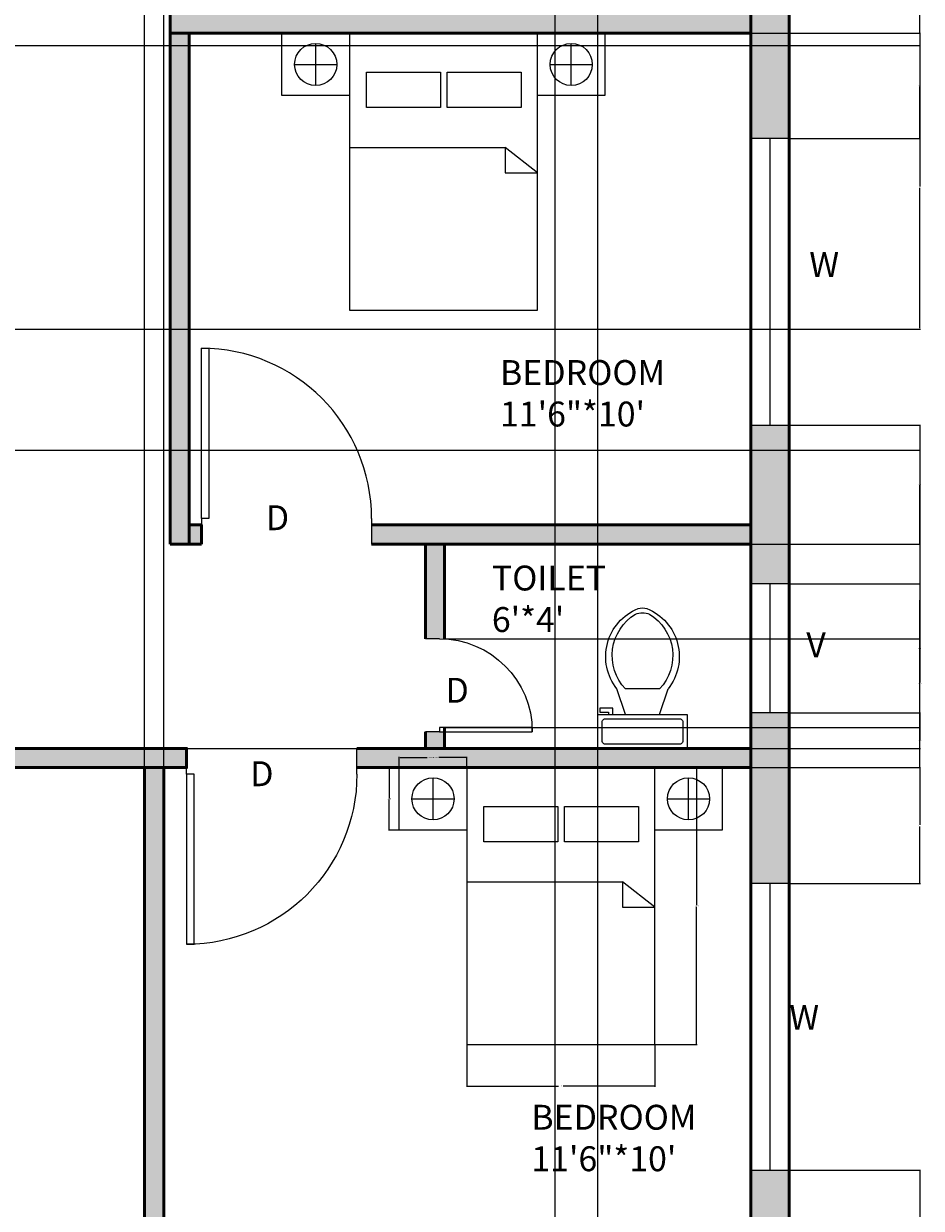
# Model space of a CAD drawing. Units: inches. Extents: x 678 to 1100, y 1432 to 2094.
# Tile 3 of 5: x 889 to 1100, y 1581 to 1860. Entities that reach past the tile are written whole.
import ezdxf

# ---------------------------------------------------------------- set-up
doc = ezdxf.new("R2010")
doc.units = ezdxf.units.IN
for name, color, linetype, lineweight in [('A-ANNO-DIMS', 2, 'Continuous', 18), ('A-AREA-IDEN', 141, 'Continuous', 25), ('A-FLOR-FIXT', 9, 'Continuous', 18), ('A-WALL-PATT', 252, 'Continuous', 13), ('DOOR', 52, 'Continuous', 25), ('FUR', 30, 'Continuous', 18), ('TEXT', 141, 'Continuous', 18), ('WALL', 140, 'Continuous', 50), ('WIND', 212, 'Continuous', 25)]:
    doc.layers.add(name, color=color, linetype=linetype, lineweight=lineweight)
doc.styles.get("Standard").update_dxf_attribs({"font": 'arial.ttf'})
doc.dimstyles.get("Standard").update_dxf_attribs({"dimtxt": 0.18, "dimasz": 0.18, "dimexe": 0.18, "dimexo": 0.0625, "dimgap": 0.09, "dimtad": 0, "dimtih": 1, "dimtoh": 1, "dimdec": 4, "dimzin": 0, "dimdsep": 46, "dimtxsty": 'Standard', "dimcen": 0.09, "dimadec": 0, "dimazin": 0, "dimtfac": 1, "dimtdec": 4, "dimtofl": 0, "dimtmove": 0, "dimatfit": 3, "dimfxl": 1, "dimtolj": 1, "dimtzin": 0, "dimarcsym": 0})

# ---------------------------------------------------------------- blocks, each defined once
blk = doc.blocks.new('*U2')
for p, q in [((0, 0), (0, -6)), ((40, 0), (40, -6))]:
    blk.add_line(p, q)
blk.add_lwpolyline([(0, 0), (0, 40), (1.75, 40), (1.75, 0)], close=True)
blk.add_arc((0, 0), 40, 0, 90)
blk = doc.blocks.new('*U4')
for p, q in [((9.5, -6), (9.5, -2)), ((-8, -8.5), (-8, -8)), ((-7, -8), (-7, -9.5)), ((-4, -8), (-6, -14)), ((4, -8), (6, -14)), ((-10, -8.5), (-8, -8.5)), ((-10, -9.5), (-10, -8.5)), ((-7, -9.5), (-10, -9.5)), ((4, -14), (-4, -14))]:
    blk.add_line(p, q)
blk.add_lwpolyline([(10.5, -8), (10.5, 0), (-10.5, 0), (-10.5, -8)], close=True)
for points in [[(-9.5, -2), (-9.5, -6)], [(8.5, -1), (-8.5, -1)], [(-8.5, -7), (8.5, -7)]]:
    blk.add_lwpolyline(points)
for centre, radius, start, end in [((-8.62, -1.88), 0.884, 81.8699, 188.1301), ((8.62, -1.88), 0.884, 351.8699, 98.1301), ((-8.62, -6.12), 0.884, 171.8699, 278.1301), ((8.62, -6.12), 0.884, 261.8699, 8.1301), ((3.52, -21.58), 12.17, 141.4691, 247.9714), ((4.2, -21.82), 11.33, 136.3677, 238.9468), ((-3.52, -21.58), 12.17, 292.0284, 38.5307), ((-4.2, -21.82), 11.33, 301.053, 43.6321), ((0, -27.88), 4, 245.7318, 294.2682), ((0, -29), 4, 254.8605, 285.1395)]:
    blk.add_arc(centre, radius, start, end)
blk = doc.blocks.new('BED')
for p, q in [((0, 38.19), (36.64, 38.19)), ((36.64, 38.19), (36.64, 32.24)), ((44.21, 32.24), (36.64, 38.19)), ((36.64, 32.24), (44.21, 32.24))]:
    blk.add_line(p, q)
for points in [[(44.21, 65.05), (0, 65.05), (0, 0), (44.21, 0)], [(4.01, 55.91), (21.41, 55.91), (21.41, 47.59), (4.01, 47.59)], [(22.97, 55.91), (40.37, 55.91), (40.37, 47.59), (22.97, 47.59)]]:
    blk.add_lwpolyline(points, close=True)
blk = doc.blocks.new('NIGHTSTAND-LAMP')
for p, q in [((7.92, 2.38), (7.92, 12.28)), ((2.97, 7.33), (12.87, 7.33))]:
    blk.add_line(p, q)
blk.add_lwpolyline([(0, 14.65), (15.83, 14.65), (15.83, 0), (0, 0)], close=True)
blk.add_circle((7.92, 7.33), 4.95)
blk = doc.blocks.new('WIN-STANDARD')
blk.add_line((4.5, 0), (4.5, 67.31))
blk.add_lwpolyline([(9, 67.31), (0, 67.31), (0, 0), (9, 0)], close=True)
blk = doc.blocks.new('*D14')
at = {"layer": 'A-ANNO-DIMS', "color": 0, "lineweight": -2, "transparency": 16777216}
for p, q in [((1037.43, 1684.93), (1047.3, 1684.93)), ((1047.12, 1684.75), (1047.12, 1652.59)), ((1047.12, 1620.06), (1047.12, 1652.22)), ((1037.43, 1619.88), (1047.3, 1619.88))]:
    blk.add_line(p, q, dxfattribs=at)
at = {"layer": 'A-ANNO-DIMS', "color": 0, "transparency": 16777216}
for points in [[(1047.09, 1684.75), (1047.15, 1684.75), (1047.12, 1684.93)], [(1047.09, 1620.06), (1047.15, 1620.06), (1047.12, 1619.88)]]:
    blk.add_solid(points, dxfattribs=at)
at = {"layer": 'Defpoints', "color": 0, "transparency": 16777216}
for p in [(1037.36, 1684.93), (1047.12, 1684.93), (1037.36, 1619.88)]:
    blk.add_point(p, dxfattribs=at)
at = {"layer": 'A-ANNO-DIMS', "color": 0, "transparency": 16777216, "insert": (1047.12, 1652.4), "char_height": 0.18, "attachment_point": 5}
blk.add_mtext('\\A1;BED 65 TYP.', dxfattribs=at)
blk = doc.blocks.new('*D15')
at = {"layer": 'A-ANNO-DIMS', "color": 0, "lineweight": -2, "transparency": 16777216}
for p, q in [((993.15, 1619.82), (993.15, 1609.94)), ((1037.36, 1619.82), (1037.36, 1609.94)), ((993.33, 1610.12), (1014.72, 1610.12)), ((1037.18, 1610.12), (1015.79, 1610.12))]:
    blk.add_line(p, q, dxfattribs=at)
at = {"layer": 'A-ANNO-DIMS', "color": 0, "transparency": 16777216}
for points in [[(993.33, 1610.15), (993.33, 1610.09), (993.15, 1610.12)], [(1037.18, 1610.15), (1037.18, 1610.09), (1037.36, 1610.12)]]:
    blk.add_solid(points, dxfattribs=at)
at = {"layer": 'Defpoints', "color": 0, "transparency": 16777216}
for p in [(993.15, 1619.88), (1037.36, 1619.88), (1037.36, 1610.12)]:
    blk.add_point(p, dxfattribs=at)
at = {"layer": 'A-ANNO-DIMS', "color": 0, "transparency": 16777216, "insert": (1015.26, 1610.12), "char_height": 0.18, "attachment_point": 5}
blk.add_mtext('\\A1;44 TYP.', dxfattribs=at)
blk = doc.blocks.new('*D16')
at = {"layer": 'A-ANNO-DIMS', "color": 0, "lineweight": -2, "transparency": 16777216}
for p, q in [((977.31, 1684.99), (977.31, 1687.48)), ((977.49, 1687.3), (983.86, 1687.3)), ((992.97, 1687.3), (986.61, 1687.3)), ((993.15, 1684.99), (993.15, 1687.48))]:
    blk.add_line(p, q, dxfattribs=at)
at = {"layer": 'A-ANNO-DIMS', "color": 0, "transparency": 16777216}
for points in [[(977.49, 1687.33), (977.49, 1687.27), (977.31, 1687.3)], [(992.97, 1687.33), (992.97, 1687.27), (993.15, 1687.3)]]:
    blk.add_solid(points, dxfattribs=at)
at = {"layer": 'Defpoints', "color": 0, "transparency": 16777216}
for p in [(993.15, 1687.3), (977.31, 1684.93), (993.15, 1684.93)]:
    blk.add_point(p, dxfattribs=at)
at = {"layer": 'A-ANNO-DIMS', "color": 0, "transparency": 16777216, "insert": (985.23, 1687.3), "char_height": 0.18, "attachment_point": 5}
blk.add_mtext('\\A1;NIGHTSTAND 16 TYP.', dxfattribs=at)
blk = doc.blocks.new('*D17')
at = {"layer": 'A-ANNO-DIMS', "color": 0, "lineweight": -2, "transparency": 16777216}
for p, q in [((977.25, 1684.93), (974.76, 1684.93)), ((974.94, 1684.75), (974.94, 1677.78)), ((974.94, 1670.45), (974.94, 1677.42)), ((977.25, 1670.27), (974.76, 1670.27))]:
    blk.add_line(p, q, dxfattribs=at)
at = {"layer": 'A-ANNO-DIMS', "color": 0, "transparency": 16777216}
for points in [[(974.91, 1684.75), (974.97, 1684.75), (974.94, 1684.93)], [(974.91, 1670.45), (974.97, 1670.45), (974.94, 1670.27)]]:
    blk.add_solid(points, dxfattribs=at)
at = {"layer": 'Defpoints', "color": 0, "transparency": 16777216}
for p in [(974.94, 1684.93), (977.31, 1684.93), (977.31, 1670.27)]:
    blk.add_point(p, dxfattribs=at)
at = {"layer": 'A-ANNO-DIMS', "color": 0, "transparency": 16777216, "insert": (974.94, 1677.6), "char_height": 0.18, "attachment_point": 5}
blk.add_mtext('\\A1;15 TYP.', dxfattribs=at)
blk = doc.blocks.new('*D33')
at = {"layer": 'A-ANNO-DIMS', "color": 0, "lineweight": -2, "transparency": 16777216}
for p, q in [((1069.02, 1590.39), (1099.79, 1590.39)), ((1099.61, 1590.21), (1099.61, 1575.59)), ((1099.61, 1560.61), (1099.61, 1575.23)), ((1069.02, 1560.43), (1099.79, 1560.43))]:
    blk.add_line(p, q, dxfattribs=at)
at = {"layer": 'A-ANNO-DIMS', "color": 0, "transparency": 16777216}
for points in [[(1099.58, 1590.21), (1099.64, 1590.21), (1099.61, 1590.39)], [(1099.58, 1560.61), (1099.64, 1560.61), (1099.61, 1560.43)]]:
    blk.add_solid(points, dxfattribs=at)
at = {"layer": 'Defpoints', "color": 0, "transparency": 16777216}
for p in [(1068.96, 1590.39), (1099.61, 1590.39), (1068.96, 1560.43)]:
    blk.add_point(p, dxfattribs=at)
at = {"layer": 'A-ANNO-DIMS', "color": 0, "transparency": 16777216, "insert": (1099.61, 1575.41), "char_height": 0.18, "attachment_point": 5}
blk.add_mtext('\\A1;29.96', dxfattribs=at)
blk = doc.blocks.new('*D34')
at = {"layer": 'A-ANNO-DIMS', "color": 0, "lineweight": -2, "transparency": 16777216}
for p, q in [((1060.02, 1684.93), (1099.79, 1684.93)), ((1099.61, 1684.75), (1099.61, 1671.5)), ((1099.61, 1657.88), (1099.61, 1671.13)), ((1069.02, 1657.7), (1099.79, 1657.7))]:
    blk.add_line(p, q, dxfattribs=at)
at = {"layer": 'A-ANNO-DIMS', "color": 0, "transparency": 16777216}
for points in [[(1099.58, 1684.75), (1099.64, 1684.75), (1099.61, 1684.93)], [(1099.58, 1657.88), (1099.64, 1657.88), (1099.61, 1657.7)]]:
    blk.add_solid(points, dxfattribs=at)
at = {"layer": 'Defpoints', "color": 0, "transparency": 16777216}
for p in [(1059.96, 1684.93), (1099.61, 1684.93), (1068.96, 1657.7)]:
    blk.add_point(p, dxfattribs=at)
at = {"layer": 'A-ANNO-DIMS', "color": 0, "transparency": 16777216, "insert": (1099.61, 1671.32), "char_height": 0.18, "attachment_point": 5}
blk.add_mtext('\\A1;27.227', dxfattribs=at)
blk = doc.blocks.new('*D35')
at = {"layer": 'A-ANNO-DIMS', "color": 0, "lineweight": -2, "transparency": 16777216}
for p, q in [((1069.02, 1697.8), (1099.79, 1697.8)), ((1099.61, 1697.62), (1099.61, 1691.55)), ((1099.61, 1685.11), (1099.61, 1691.18)), ((1060.02, 1684.93), (1099.79, 1684.93))]:
    blk.add_line(p, q, dxfattribs=at)
at = {"layer": 'A-ANNO-DIMS', "color": 0, "transparency": 16777216}
for points in [[(1099.58, 1697.62), (1099.64, 1697.62), (1099.61, 1697.8)], [(1099.58, 1685.11), (1099.64, 1685.11), (1099.61, 1684.93)]]:
    blk.add_solid(points, dxfattribs=at)
at = {"layer": 'Defpoints', "color": 0, "transparency": 16777216}
for p in [(1068.96, 1697.8), (1099.61, 1697.8), (1059.96, 1684.93)]:
    blk.add_point(p, dxfattribs=at)
at = {"layer": 'A-ANNO-DIMS', "color": 0, "transparency": 16777216, "insert": (1099.61, 1691.37), "char_height": 0.18, "attachment_point": 5}
blk.add_mtext('\\A1;12.873', dxfattribs=at)
blk = doc.blocks.new('*D36')
at = {"layer": 'A-ANNO-DIMS', "color": 0, "lineweight": -2, "transparency": 16777216}
for p, q in [((1069.02, 1728.14), (1099.79, 1728.14)), ((1099.61, 1727.96), (1099.61, 1713.16)), ((1099.61, 1697.98), (1099.61, 1712.79)), ((1069.02, 1697.8), (1099.79, 1697.8))]:
    blk.add_line(p, q, dxfattribs=at)
at = {"layer": 'A-ANNO-DIMS', "color": 0, "transparency": 16777216}
for points in [[(1099.58, 1727.96), (1099.64, 1727.96), (1099.61, 1728.14)], [(1099.58, 1697.98), (1099.64, 1697.98), (1099.61, 1697.8)]]:
    blk.add_solid(points, dxfattribs=at)
at = {"layer": 'Defpoints', "color": 0, "transparency": 16777216}
for p in [(1068.96, 1728.14), (1099.61, 1728.14), (1068.96, 1697.8)]:
    blk.add_point(p, dxfattribs=at)
at = {"layer": 'A-ANNO-DIMS', "color": 0, "transparency": 16777216, "insert": (1099.61, 1712.97), "char_height": 0.18, "attachment_point": 5}
blk.add_mtext('\\A1;30.34', dxfattribs=at)
blk = doc.blocks.new('*D37')
at = {"layer": 'A-ANNO-DIMS', "color": 0, "lineweight": -2, "transparency": 16777216}
for p, q in [((1069.02, 1765.41), (1099.79, 1765.41)), ((1099.61, 1765.23), (1099.61, 1751.6)), ((1099.61, 1737.61), (1099.61, 1751.24)), ((1060.02, 1737.43), (1099.79, 1737.43))]:
    blk.add_line(p, q, dxfattribs=at)
at = {"layer": 'A-ANNO-DIMS', "color": 0, "transparency": 16777216}
for points in [[(1099.58, 1765.23), (1099.64, 1765.23), (1099.61, 1765.41)], [(1099.58, 1737.61), (1099.64, 1737.61), (1099.61, 1737.43)]]:
    blk.add_solid(points, dxfattribs=at)
at = {"layer": 'Defpoints', "color": 0, "transparency": 16777216}
for p in [(1068.96, 1765.41), (1099.61, 1765.41), (1059.96, 1737.43)]:
    blk.add_point(p, dxfattribs=at)
at = {"layer": 'A-ANNO-DIMS', "color": 0, "transparency": 16777216, "insert": (1099.61, 1751.42), "char_height": 0.18, "attachment_point": 5}
blk.add_mtext('\\A1;27.98', dxfattribs=at)
blk = doc.blocks.new('*D38')
at = {"layer": 'A-ANNO-DIMS', "color": 0, "lineweight": -2, "transparency": 16777216}
for p, q in [((1060.02, 1857.43), (1099.79, 1857.43)), ((1099.61, 1857.25), (1099.61, 1845.25)), ((1099.61, 1832.9), (1099.61, 1844.89)), ((1069.02, 1832.72), (1099.79, 1832.72))]:
    blk.add_line(p, q, dxfattribs=at)
at = {"layer": 'A-ANNO-DIMS', "color": 0, "transparency": 16777216}
for points in [[(1099.58, 1857.25), (1099.64, 1857.25), (1099.61, 1857.43)], [(1099.58, 1832.9), (1099.64, 1832.9), (1099.61, 1832.72)]]:
    blk.add_solid(points, dxfattribs=at)
at = {"layer": 'Defpoints', "color": 0, "transparency": 16777216}
for p in [(1059.96, 1857.43), (1099.61, 1857.43), (1068.96, 1832.72)]:
    blk.add_point(p, dxfattribs=at)
at = {"layer": 'A-ANNO-DIMS', "color": 0, "transparency": 16777216, "insert": (1099.61, 1845.07), "char_height": 0.18, "attachment_point": 5}
blk.add_mtext('\\A1;24.71', dxfattribs=at)
blk = doc.blocks.new('*D39')
at = {"layer": 'A-ANNO-DIMS', "color": 0, "lineweight": -2, "transparency": 16777216}
for p, q in [((1069.02, 1935.32), (1099.79, 1935.32)), ((1099.61, 1935.14), (1099.61, 1896.56)), ((1099.61, 1857.61), (1099.61, 1896.19)), ((1060.02, 1857.43), (1099.79, 1857.43))]:
    blk.add_line(p, q, dxfattribs=at)
at = {"layer": 'A-ANNO-DIMS', "color": 0, "transparency": 16777216}
for points in [[(1099.58, 1935.14), (1099.64, 1935.14), (1099.61, 1935.32)], [(1099.58, 1857.61), (1099.64, 1857.61), (1099.61, 1857.43)]]:
    blk.add_solid(points, dxfattribs=at)
at = {"layer": 'Defpoints', "color": 0, "transparency": 16777216}
for p in [(1068.96, 1935.32), (1099.61, 1935.32), (1059.96, 1857.43)]:
    blk.add_point(p, dxfattribs=at)
at = {"layer": 'A-ANNO-DIMS', "color": 0, "transparency": 16777216, "insert": (1099.61, 1896.38), "char_height": 0.18, "attachment_point": 5}
blk.add_mtext('\\A1;77.9', dxfattribs=at)
blk = doc.blocks.new('*D41')
at = {"layer": 'A-ANNO-DIMS', "color": 0, "lineweight": -2, "transparency": 16777216}
for p, q in [((718.02, 1759.52), (1099.79, 1759.52)), ((1099.61, 1759.34), (1099.61, 1724.66)), ((1099.61, 1689.61), (1099.61, 1724.29)), ((718.02, 1689.43), (1099.79, 1689.43))]:
    blk.add_line(p, q, dxfattribs=at)
at = {"layer": 'A-ANNO-DIMS', "color": 0, "transparency": 16777216}
for points in [[(1099.58, 1759.34), (1099.64, 1759.34), (1099.61, 1759.52)], [(1099.58, 1689.61), (1099.64, 1689.61), (1099.61, 1689.43)]]:
    blk.add_solid(points, dxfattribs=at)
at = {"layer": 'Defpoints', "color": 0, "transparency": 16777216}
for p in [(717.96, 1759.52), (1099.61, 1759.52), (717.96, 1689.43)]:
    blk.add_point(p, dxfattribs=at)
at = {"layer": 'A-ANNO-DIMS', "color": 0, "transparency": 16777216, "insert": (1099.61, 1724.48), "char_height": 0.18, "attachment_point": 5}
blk.add_mtext('\\A1;70.1', dxfattribs=at)
blk = doc.blocks.new('*D46')
at = {"layer": 'A-ANNO-DIMS', "color": 0, "lineweight": -2, "transparency": 16777216}
for p, q in [((988.02, 1715.16), (1099.79, 1715.16)), ((1099.61, 1714.98), (1099.61, 1704.92)), ((1099.61, 1694.5), (1099.61, 1704.56)), ((988.02, 1694.32), (1099.79, 1694.32))]:
    blk.add_line(p, q, dxfattribs=at)
at = {"layer": 'A-ANNO-DIMS', "color": 0, "transparency": 16777216}
for points in [[(1099.58, 1714.98), (1099.64, 1714.98), (1099.61, 1715.16)], [(1099.58, 1694.5), (1099.64, 1694.5), (1099.61, 1694.32)]]:
    blk.add_solid(points, dxfattribs=at)
at = {"layer": 'Defpoints', "color": 0, "transparency": 16777216}
for p in [(987.96, 1715.16), (1099.61, 1715.16), (987.96, 1694.32)]:
    blk.add_point(p, dxfattribs=at)
at = {"layer": 'A-ANNO-DIMS', "color": 0, "transparency": 16777216, "insert": (1099.61, 1704.74), "char_height": 0.18, "attachment_point": 5}
blk.add_mtext('\\A1;20.844', dxfattribs=at)
blk = doc.blocks.new('*D48')
at = {"layer": 'A-ANNO-DIMS', "color": 0, "lineweight": -2, "transparency": 16777216}
for p, q in [((917.46, 1560.49), (917.46, 2093.76)), ((917.64, 2093.58), (919.45, 2093.58)), ((921.78, 2093.58), (919.97, 2093.58)), ((921.96, 1560.49), (921.96, 2093.76))]:
    blk.add_line(p, q, dxfattribs=at)
at = {"layer": 'A-ANNO-DIMS', "color": 0, "transparency": 16777216}
for points in [[(917.64, 2093.61), (917.64, 2093.55), (917.46, 2093.58)], [(921.78, 2093.61), (921.78, 2093.55), (921.96, 2093.58)]]:
    blk.add_solid(points, dxfattribs=at)
at = {"layer": 'Defpoints', "color": 0, "transparency": 16777216}
for p in [(921.96, 2093.58), (917.46, 1560.43), (921.96, 1560.43)]:
    blk.add_point(p, dxfattribs=at)
at = {"layer": 'A-ANNO-DIMS', "color": 0, "transparency": 16777216, "insert": (919.71, 2093.58), "char_height": 0.18, "attachment_point": 5}
blk.add_mtext('\\A1;4.5', dxfattribs=at)
blk = doc.blocks.new('*D49')
at = {"layer": 'A-ANNO-DIMS', "color": 0, "lineweight": -2, "transparency": 16777216}
for p, q in [((1013.96, 1471.99), (1013.96, 2093.76)), ((1014.14, 2093.58), (1018.75, 2093.58)), ((1023.78, 2093.58), (1019.17, 2093.58)), ((1023.96, 1471.99), (1023.96, 2093.76))]:
    blk.add_line(p, q, dxfattribs=at)
at = {"layer": 'A-ANNO-DIMS', "color": 0, "transparency": 16777216}
for points in [[(1014.14, 2093.61), (1014.14, 2093.55), (1013.96, 2093.58)], [(1023.78, 2093.61), (1023.78, 2093.55), (1023.96, 2093.58)]]:
    blk.add_solid(points, dxfattribs=at)
at = {"layer": 'Defpoints', "color": 0, "transparency": 16777216}
for p in [(1023.96, 2093.58), (1013.96, 1471.93), (1023.96, 1471.93)]:
    blk.add_point(p, dxfattribs=at)
at = {"layer": 'A-ANNO-DIMS', "color": 0, "transparency": 16777216, "insert": (1018.96, 2093.58), "char_height": 0.18, "attachment_point": 5}
blk.add_mtext('\\A1;10', dxfattribs=at)
blk = doc.blocks.new('*D50')
at = {"layer": 'A-ANNO-DIMS', "color": 0, "lineweight": -2, "transparency": 16777216}
for p, q in [((1023.96, 1471.99), (1023.96, 2093.76)), ((1024.14, 2093.58), (1041.74, 2093.58)), ((1059.78, 2093.58), (1042.18, 2093.58)), ((1059.96, 1471.99), (1059.96, 2093.76))]:
    blk.add_line(p, q, dxfattribs=at)
at = {"layer": 'A-ANNO-DIMS', "color": 0, "transparency": 16777216}
for points in [[(1024.14, 2093.61), (1024.14, 2093.55), (1023.96, 2093.58)], [(1059.78, 2093.61), (1059.78, 2093.55), (1059.96, 2093.58)]]:
    blk.add_solid(points, dxfattribs=at)
at = {"layer": 'Defpoints', "color": 0, "transparency": 16777216}
for p in [(1059.96, 2093.58), (1023.96, 1471.93), (1059.96, 1471.93)]:
    blk.add_point(p, dxfattribs=at)
at = {"layer": 'A-ANNO-DIMS', "color": 0, "transparency": 16777216, "insert": (1041.96, 2093.58), "char_height": 0.18, "attachment_point": 5}
blk.add_mtext('\\A1;36', dxfattribs=at)
blk = doc.blocks.new('*D56')
at = {"layer": 'A-ANNO-DIMS', "color": 0, "lineweight": -2, "transparency": 16777216}
for p, q in [((720.28, 1854.56), (1099.79, 1854.56)), ((1099.61, 1854.38), (1099.61, 1821.43)), ((1099.61, 1788.12), (1099.61, 1821.06)), ((720.28, 1787.94), (1099.79, 1787.94))]:
    blk.add_line(p, q, dxfattribs=at)
at = {"layer": 'A-ANNO-DIMS', "color": 0, "transparency": 16777216}
for points in [[(1099.58, 1854.38), (1099.64, 1854.38), (1099.61, 1854.56)], [(1099.58, 1788.12), (1099.64, 1788.12), (1099.61, 1787.94)]]:
    blk.add_solid(points, dxfattribs=at)
at = {"layer": 'Defpoints', "color": 0, "transparency": 16777216}
for p in [(720.22, 1854.56), (1099.61, 1854.56), (720.22, 1787.94)]:
    blk.add_point(p, dxfattribs=at)
at = {"layer": 'A-ANNO-DIMS', "color": 0, "transparency": 16777216, "insert": (1099.61, 1821.25), "char_height": 0.18, "attachment_point": 5}
blk.add_mtext('\\A1;66.62', dxfattribs=at)

msp = doc.modelspace()

# ---------------------------------------------------------------- hatches: boundary and pattern name
at = {"layer": 'A-WALL-PATT'}
h = msp.add_hatch(color=256, dxfattribs=at)
h.dxf.hatch_style = 1
h.paths.add_polyline_path([(859.7133, 2062.9286), (708.9606, 2062.9286), (708.9606, 2031.3203), (717.9606, 2031.3203), (717.9606, 2053.9286), (837.9606, 2053.9286), (859.7133, 2053.9286)])
h.paths.add_polyline_path([(957.0069, 2062.9286), (896.0724, 2062.9286), (896.0724, 2053.9286), (957.0069, 2053.9286)])
h.paths.add_polyline_path([(842.4606, 2053.9286), (837.9606, 2053.9286), (837.9606, 2005.4286), (842.4606, 2005.4286), (923.4606, 2005.4286), (923.4606, 2009.9286), (842.4606, 2009.9286)])
h.paths.add_polyline_path([(927.9606, 2053.9286), (923.4606, 2053.9286), (923.4606, 2052.1286), (924.8103, 2052.1286), (927.9606, 2052.1286)])
h.paths.add_polyline_path([(1068.9606, 2062.9286), (1024.3184, 2062.9286), (1024.3184, 2053.9286), (1028.6041, 2053.9286), (1059.9606, 2053.9286), (1059.9606, 2002.6361), (1068.9606, 2002.6361)])
h.paths.add_polyline_path([(1059.9606, 1861.9286), (996.9604, 1861.9286), (927.9606, 1861.9286), (923.4606, 1861.9286), (923.4606, 1857.4286), (1059.9606, 1857.4286)], flags=17)
h.paths.add_polyline_path([(927.9606, 2031.1269), (924.8103, 2031.1269, -0.01607952), (923.4606, 2031.1703), (923.4606, 1905.3856), (927.9606, 1905.3856)])
h.paths.add_polyline_path([(923.4606, 1957.9286), (842.4606, 1957.9286), (842.4606, 1969.339), (837.9606, 1969.339), (837.9606, 1953.4286), (923.4606, 1953.4286)])
h.paths.add_polyline_path([(774.6357, 1957.9286), (717.9606, 1957.9286), (717.9606, 1953.4286), (774.6357, 1953.4286)])
h.paths.add_polyline_path([(717.9606, 1979.9404), (708.9606, 1979.9404), (708.9606, 1945.1463), (717.9606, 1945.1463)])
h.paths.add_polyline_path([(840.5596, 1861.9286), (717.9606, 1861.9286), (717.9606, 1857.4286), (840.5596, 1857.4286)], flags=17)
h.paths.add_polyline_path([(927.9606, 1865.3856), (923.4606, 1865.3856), (923.4606, 1861.9286), (927.9606, 1861.9286)], flags=17)
h.paths.add_polyline_path([(1059.9606, 1689.4286), (967.3461, 1689.4286), (967.3461, 1684.9286), (1059.9606, 1684.9286)], flags=17)
h.paths.add_polyline_path([(987.9606, 1737.4286), (983.4606, 1737.4286), (983.4606, 1715.196), (986.7357, 1715.196, -0.01403382), (987.9606, 1715.1616)], flags=17)
h.paths.add_polyline_path([(916.0499, 2036.8414), (924.8721, 2036.8414), (924.8721, 2048.8901), (916.0499, 2048.8901)], flags=9)
h.paths.add_polyline_path([(921.7778, 1883.2914), (930.5999, 1883.2914), (930.5999, 1895.3401), (921.7778, 1895.3401)], flags=25)
h.paths.add_polyline_path([(732.1085, 1683.0506), (740.9307, 1683.0506), (740.9307, 1695.0993), (732.1085, 1695.0993)], flags=25)
h.paths.add_polyline_path([(943.8458, 1737.5114), (952.6679, 1737.5114), (952.6679, 1749.5601), (943.8458, 1749.5601)], flags=25)
h.paths.add_polyline_path([(986.0751, 1696.9795), (994.8973, 1696.9795), (994.8973, 1709.0282), (986.0751, 1709.0282)], flags=25)
h.paths.add_polyline_path([(940.1881, 1677.378), (949.0103, 1677.378), (949.0103, 1689.4267), (940.1881, 1689.4267)], flags=25)
h.paths.add_polyline_path([(998.6262, 1761.7469), (1044.0453, 1761.7469), (1044.0453, 1783.5644), (998.6262, 1783.5644)], flags=25)
h.paths.add_polyline_path([(997.3001, 1713.4735), (1028.9316, 1713.4735), (1028.9316, 1735.2909), (997.3001, 1735.2909)], flags=25)
h.paths.add_polyline_path([(1005.9896, 1586.8139), (1051.4087, 1586.8139), (1051.4087, 1608.6313), (1005.9896, 1608.6313)], flags=25)
h.paths.add_polyline_path([(794.7038, 1552.8124), (873.8721, 1552.8124), (873.8721, 1574.6298), (794.7038, 1574.6298)], flags=25)
h.paths.add_polyline_path([(774.2693, 1771.1228), (831.9444, 1771.1228), (831.9444, 1792.9403), (774.2693, 1792.9403)], flags=25)
h.paths.add_polyline_path([(750.0357, 1897.1514), (786.4291, 1897.1514), (786.4291, 1918.9689), (750.0357, 1918.9689)], flags=25)
h.paths.add_polyline_path([(974.9086, 1953.7921), (1020.3276, 1953.7921), (1020.3276, 1975.6096), (974.9086, 1975.6096)], flags=9)
h.paths.add_polyline_path([(859.1564, 1973.8092), (890.2175, 1973.8092), (890.2175, 1995.6267), (859.1564, 1995.6267)], flags=9)
h.paths.add_polyline_path([(753.2305, 1989.0219), (792.2962, 1989.0219), (792.2962, 2010.8393), (753.2305, 2010.8393)], flags=9)
h.paths.add_polyline_path([(1067.3992, 1620.1515), (1078.032, 1620.1515), (1078.032, 1632.2002), (1067.3992, 1632.2002)], flags=9)
h.paths.add_polyline_path([(846.8446, 2028.8178), (878.5079, 2028.8178), (878.5079, 2050.6353), (846.8446, 2050.6353)], flags=25)
h.paths.add_polyline_path([(1059.9606, 1832.7202), (1068.9606, 1832.7202), (1068.9606, 1935.3246), (1059.9606, 1935.3246)])
h.paths.add_polyline_path([(1068.9606, 1765.4088), (1059.9606, 1765.4088), (1059.9606, 1728.1446), (1068.9606, 1728.1446)])
h.paths.add_polyline_path([(1059.9606, 1657.7018), (1068.9606, 1657.7018), (1068.9606, 1697.8017), (1059.9606, 1697.8017)])
h.paths.add_polyline_path([(1068.9606, 1590.3903), (1059.9606, 1590.3903), (1059.9606, 1551.1623), (1068.9606, 1551.1623)])
h.paths.add_polyline_path([(708.9606, 1826.8331), (717.9606, 1826.8331), (717.9606, 1877.8348), (708.9606, 1877.8348)])
h.paths.add_polyline_path([(717.9606, 1759.5217), (708.9606, 1759.5217), (708.9606, 1462.9286), (1068.9606, 1462.9286), (1068.9606, 1483.8508), (1059.9606, 1483.8508), (1059.9606, 1471.9286), (717.9606, 1471.9286)])
h = msp.add_hatch(color=256, dxfattribs=at)
h.dxf.hatch_style = 1
h.paths.add_polyline_path([(1059.9606, 1741.9286), (970.7942, 1741.9286), (970.7942, 1737.4286), (1059.9606, 1737.4286)])
h.paths.add_polyline_path([(927.3461, 1689.4286), (759.4099, 1689.4286), (759.4099, 1684.9286), (927.3461, 1684.9286)])
h.paths.add_polyline_path([(921.9606, 1684.9286), (917.4606, 1684.9286), (917.4606, 1560.4286), (921.9606, 1560.4286)])
h.paths.add_polyline_path([(1059.9606, 1564.9286), (921.9606, 1564.9286), (921.9606, 1560.4286), (1059.9606, 1560.4286)])
h.paths.add_polyline_path([(916.0499, 2036.8414), (924.8721, 2036.8414), (924.8721, 2048.8901), (916.0499, 2048.8901)], flags=9)
h.paths.add_polyline_path([(921.7778, 1883.2914), (930.5999, 1883.2914), (930.5999, 1895.3401), (921.7778, 1895.3401)], flags=9)
h.paths.add_polyline_path([(732.1085, 1683.0506), (740.9307, 1683.0506), (740.9307, 1695.0993), (732.1085, 1695.0993)], flags=9)
h.paths.add_polyline_path([(943.8458, 1737.5114), (952.6679, 1737.5114), (952.6679, 1749.5601), (943.8458, 1749.5601)], flags=9)
h.paths.add_polyline_path([(986.0751, 1696.9795), (994.8973, 1696.9795), (994.8973, 1709.0282), (986.0751, 1709.0282)], flags=9)
h.paths.add_polyline_path([(940.1881, 1677.378), (949.0103, 1677.378), (949.0103, 1689.4267), (940.1881, 1689.4267)], flags=9)
h.paths.add_polyline_path([(998.6262, 1761.7469), (1044.0453, 1761.7469), (1044.0453, 1783.5644), (998.6262, 1783.5644)], flags=9)
h.paths.add_polyline_path([(1005.9896, 1586.8139), (1051.4087, 1586.8139), (1051.4087, 1608.6313), (1005.9896, 1608.6313)], flags=9)
h.paths.add_polyline_path([(794.7038, 1552.8124), (873.8721, 1552.8124), (873.8721, 1574.6298), (794.7038, 1574.6298)], flags=9)
h.paths.add_polyline_path([(774.2693, 1771.1228), (831.9444, 1771.1228), (831.9444, 1792.9403), (774.2693, 1792.9403)], flags=9)
h.paths.add_polyline_path([(750.0357, 1897.1514), (786.4291, 1897.1514), (786.4291, 1918.9689), (750.0357, 1918.9689)], flags=9)
h.paths.add_polyline_path([(974.9086, 1953.7921), (1020.3276, 1953.7921), (1020.3276, 1975.6096), (974.9086, 1975.6096)], flags=9)
h.paths.add_polyline_path([(859.1564, 1973.8092), (890.2175, 1973.8092), (890.2175, 1995.6267), (859.1564, 1995.6267)], flags=9)
h.paths.add_polyline_path([(846.8446, 2028.8178), (878.5079, 2028.8178), (878.5079, 2050.6353), (846.8446, 2050.6353)], flags=9)
h.paths.add_polyline_path([(753.2305, 1989.0219), (792.2962, 1989.0219), (792.2962, 2010.8393), (753.2305, 2010.8393)], flags=9)
h = msp.add_hatch(color=256, dxfattribs=at)
h.dxf.hatch_style = 1
h.paths.add_polyline_path([(927.9606, 1857.4286), (923.4606, 1857.4286), (923.4606, 1737.4286), (927.9606, 1737.4286)])
h.paths.add_polyline_path([(930.7942, 1741.9286), (927.9606, 1741.9286), (927.9606, 1737.4286), (930.7942, 1737.4286)])
h.paths.add_polyline_path([(916.0499, 2036.8414), (924.8721, 2036.8414), (924.8721, 2048.8901), (916.0499, 2048.8901)], flags=9)
h.paths.add_polyline_path([(921.7778, 1883.2914), (930.5999, 1883.2914), (930.5999, 1895.3401), (921.7778, 1895.3401)], flags=9)
h.paths.add_polyline_path([(732.1085, 1683.0506), (740.9307, 1683.0506), (740.9307, 1695.0993), (732.1085, 1695.0993)], flags=9)
h.paths.add_polyline_path([(943.8458, 1737.5114), (952.6679, 1737.5114), (952.6679, 1749.5601), (943.8458, 1749.5601)], flags=9)
h.paths.add_polyline_path([(986.0751, 1696.9795), (994.8973, 1696.9795), (994.8973, 1709.0282), (986.0751, 1709.0282)], flags=9)
h.paths.add_polyline_path([(940.1881, 1677.378), (949.0103, 1677.378), (949.0103, 1689.4267), (940.1881, 1689.4267)], flags=9)
h.paths.add_polyline_path([(998.6262, 1761.7469), (1044.0453, 1761.7469), (1044.0453, 1783.5644), (998.6262, 1783.5644)], flags=9)
h.paths.add_polyline_path([(997.3001, 1713.4735), (1028.9316, 1713.4735), (1028.9316, 1735.2909), (997.3001, 1735.2909)], flags=9)
h.paths.add_polyline_path([(1005.9896, 1586.8139), (1051.4087, 1586.8139), (1051.4087, 1608.6313), (1005.9896, 1608.6313)], flags=9)
h.paths.add_polyline_path([(794.7038, 1552.8124), (873.8721, 1552.8124), (873.8721, 1574.6298), (794.7038, 1574.6298)], flags=9)
h.paths.add_polyline_path([(774.2693, 1771.1228), (831.9444, 1771.1228), (831.9444, 1792.9403), (774.2693, 1792.9403)], flags=9)
h.paths.add_polyline_path([(750.0357, 1897.1514), (786.4291, 1897.1514), (786.4291, 1918.9689), (750.0357, 1918.9689)], flags=9)
h.paths.add_polyline_path([(974.9086, 1953.7921), (1020.3276, 1953.7921), (1020.3276, 1975.6096), (974.9086, 1975.6096)], flags=9)
h.paths.add_polyline_path([(859.1564, 1973.8092), (890.2175, 1973.8092), (890.2175, 1995.6267), (859.1564, 1995.6267)], flags=9)
h.paths.add_polyline_path([(846.8446, 2028.8178), (878.5079, 2028.8178), (878.5079, 2050.6353), (846.8446, 2050.6353)], flags=9)
h.paths.add_polyline_path([(753.2305, 1989.0219), (792.2962, 1989.0219), (792.2962, 2010.8393), (753.2305, 2010.8393)], flags=9)
h = msp.add_hatch(color=256, dxfattribs=at)
h.dxf.hatch_style = 1
h.paths.add_polyline_path([(987.9606, 1693.3622), (986.7357, 1693.3622), (983.4606, 1693.3622), (983.4606, 1689.4286), (987.9606, 1689.4286)])

# ---------------------------------------------------------------- linework, layer by layer
at = {"layer": 'WALL'}
for p, q in [((1068.9606, 2062.9286), (1068.9606, 1462.9286)), ((923.4606, 1865.3856), (923.4606, 1857.4286)), ((923.4606, 1857.4286), (1059.9606, 1857.4286)), ((923.4606, 1857.4286), (923.4606, 1737.4286)), ((927.9606, 1857.4286), (927.9606, 1741.9286)), ((1059.9606, 1857.4286), (1059.9606, 1737.4286)), ((1059.9606, 1857.4286), (1059.9606, 1737.4286)), ((930.7942, 1741.9286), (927.9606, 1741.9286)), ((1059.9606, 1741.9286), (970.7942, 1741.9286)), ((930.7942, 1737.4286), (923.4606, 1737.4286)), ((1059.9606, 1737.4286), (970.7942, 1737.4286)), ((983.4606, 1715.196), (983.4606, 1737.4286)), ((987.9606, 1715.1616), (987.9606, 1737.4286)), ((1059.9606, 1737.4286), (1059.9606, 1689.4286)), ((983.4606, 1689.4286), (983.4606, 1693.3622)), ((987.9606, 1689.4286), (987.9606, 1694.3174)), ((917.4606, 1689.4286), (759.4099, 1689.4286)), ((927.3461, 1689.4286), (917.4606, 1689.4286)), ((1059.9606, 1689.4286), (967.3461, 1689.4286)), ((1059.9606, 1689.4286), (987.9606, 1689.4286)), ((921.9606, 1684.9286), (759.4099, 1684.9286)), ((917.4606, 1684.9286), (917.4606, 1560.4286)), ((921.9606, 1684.9286), (921.9606, 1564.9286)), ((927.3461, 1684.9286), (921.9606, 1684.9286)), ((1059.9606, 1684.9286), (967.3461, 1684.9286)), ((1059.9606, 1684.9286), (983.4606, 1684.9286))]:
    msp.add_line(p, q, dxfattribs=at)
for points in [[(708.9606, 2062.9286), (1068.9606, 2062.9286), (1068.9606, 1462.9286), (708.9606, 1462.9286)], [(717.9606, 2053.9286), (1059.9606, 2053.9286), (1059.9606, 1471.9286), (717.9606, 1471.9286)], [(923.4606, 1737.4286), (927.9606, 1737.4286), (927.9606, 1857.4286), (923.4606, 1857.4286)], [(930.7942, 1737.4286), (927.9606, 1737.4286), (927.9606, 1741.9286), (930.7942, 1741.9286)], [(759.4099, 1684.9286), (927.3461, 1684.9286), (927.3461, 1689.4286), (759.4099, 1689.4286)], [(917.4606, 1560.4286), (921.9606, 1560.4286), (921.9606, 1684.9286), (917.4606, 1684.9286)]]:
    msp.add_lwpolyline(points, close=True, dxfattribs=at)
at = {"layer": 'WIND'}
msp.add_line((1064.4606, 1697.8017), (1064.4606, 1728.1446), dxfattribs=at)
msp.add_lwpolyline([(1059.9606, 1728.1446), (1068.9606, 1728.1446), (1068.9606, 1697.8017), (1059.9606, 1697.8017)], close=True, dxfattribs=at)

# ---------------------------------------------------------------- block references
at = {"layer": 'A-FLOR-FIXT', "xscale": -1, "rotation": 180}
msp.add_blockref('*U4', (1034.4606, 1689.4286), dxfattribs=at)
at = {"layer": 'DOOR'}
msp.add_blockref('*U2', (930.7942, 1743.4286), dxfattribs=at)
at = {"layer": 'DOOR', "xscale": -0.5458459510788223, "yscale": 0.5458459510788223, "zscale": 0.5458459510788223, "rotation": 270}
msp.add_blockref('*U2', (986.7357, 1693.3622), dxfattribs=at)
at = {"layer": 'DOOR', "xscale": -1, "rotation": 180}
msp.add_blockref('*U2', (927.3461, 1683.4286), dxfattribs=at)
at = {"layer": 'FUR'}
for name, p in [('NIGHTSTAND-LAMP', (949.7481, 1842.774)), ('BED', (965.5822, 1792.379)), ('NIGHTSTAND-LAMP', (1009.7962, 1842.774)), ('NIGHTSTAND-LAMP', (977.3149, 1670.274)), ('BED', (993.149, 1619.879)), ('NIGHTSTAND-LAMP', (1037.363, 1670.274))]:
    msp.add_blockref(name, p, dxfattribs=at)
at = {"layer": 'WIND'}
for p in [(1059.961, 1765.4089), (1059.961, 1590.3905)]:
    msp.add_blockref('WIN-STANDARD', p, dxfattribs=at)

# ---------------------------------------------------------------- texts
at = {"layer": 'A-AREA-IDEN', "char_height": 5.84689, "attachment_point": 1}
for s, insert in [('BEDROOM\\P11\'6"*10\'', (1000.9774, 1780.6589)), ("TOILET\\P6'*4'", (999.069, 1732.3854)), ('BEDROOM\\P11\'6"*10\'', (1008.3407, 1605.7258))]:
    msp.add_mtext_dynamic_manual_height_columns(s, width=180.890738, gutter_width=29.2344, heights=[0], dxfattribs=dict(at, insert=insert))
at = {"layer": 'TEXT', "char_height": 5.8469, "attachment_point": 1}
for s, insert in [('W', (1073.6549, 1806.0397)), ('D', (945.9376, 1746.5509)), ('V', (1072.9523, 1716.6944)), ('D', (988.167, 1706.019)), ('D', (942.28, 1686.4176)), ('W', (1068.9606, 1629.191))]:
    msp.add_mtext_dynamic_manual_height_columns(s, width=180.890738, gutter_width=29.2344, heights=[0], dxfattribs=dict(at, insert=insert))

# ---------------------------------------------------------------- dimensions: what is measured, and where the dimension line sits
at = {"layer": 'A-ANNO-DIMS'}
for base, p1, p2, override, picture, middle in [((921.9606, 2093.5786), (917.4606, 1560.4286), (921.9606, 1560.4286), {"dimdec": 1, "dimlfac": 1, "dimrnd": 0, "dimzin": 0, "dimdsep": 46, "dimlunit": 2}, '*D48', (919.7106, 2093.5786)), ((1023.9606, 2093.5786), (1013.9606, 1471.9286), (1023.9606, 1471.9286), {"dimdec": 0, "dimlfac": 1, "dimrnd": 0, "dimzin": 0, "dimdsep": 46, "dimlunit": 2}, '*D49', (1018.9606, 2093.5786)), ((1059.9606, 2093.5786), (1023.9606, 1471.9286), (1059.9606, 1471.9286), {"dimdec": 0, "dimlfac": 1, "dimrnd": 0, "dimzin": 0, "dimdsep": 46, "dimlunit": 2}, '*D50', (1041.9606, 2093.5786))]:
    dim = msp.add_linear_dim(base=base, p1=p1, p2=p2, dimstyle='Standard', override=override, dxfattribs=at)
    dim.commit()
    dim.dimension.update_dxf_attribs({"geometry": picture, "text_midpoint": middle})
for base, p1, p2, override, picture, middle in [((1099.6106, 1935.3246), (1059.9606, 1857.4286), (1068.9606, 1935.3246), {"dimdec": 1, "dimlfac": 1, "dimrnd": 0, "dimzin": 0, "dimdsep": 46, "dimlunit": 2}, '*D39', (1099.6106, 1896.3766)), ((1099.6106, 1857.4286), (1068.9606, 1832.7202), (1059.9606, 1857.4286), {"dimdec": 2, "dimlfac": 1, "dimrnd": 0, "dimzin": 0, "dimdsep": 46, "dimlunit": 2}, '*D38', (1099.6106, 1845.0744)), ((1099.6106, 1854.5558), (720.2201, 1787.9351), (720.2201, 1854.5558), {"dimdec": 2, "dimlfac": 1, "dimrnd": 0, "dimzin": 0, "dimdsep": 46, "dimlunit": 2}, '*D56', (1099.6106, 1821.2455)), ((1099.6106, 1765.4088), (1059.9606, 1737.4286), (1068.9606, 1765.4088), {"dimdec": 2, "dimlfac": 1, "dimrnd": 0, "dimzin": 0, "dimdsep": 46, "dimlunit": 2}, '*D37', (1099.6106, 1751.4187)), ((1099.6106, 1759.5217), (717.9606, 1689.4286), (717.9606, 1759.5217), {"dimdec": 1, "dimlfac": 1, "dimrnd": 0, "dimzin": 0, "dimdsep": 46, "dimlunit": 2}, '*D41', (1099.6106, 1724.4751)), ((1099.6106, 1728.1446), (1068.9606, 1697.8017), (1068.9606, 1728.1446), {"dimdec": 2, "dimlfac": 1, "dimrnd": 0, "dimzin": 0, "dimdsep": 46, "dimlunit": 2}, '*D36', (1099.6106, 1712.9732)), ((1099.6106, 1715.1616), (987.9606, 1694.3174), (987.9606, 1715.1616), {"dimdec": 3, "dimlfac": 1, "dimrnd": 0, "dimzin": 0, "dimdsep": 46, "dimlunit": 2}, '*D46', (1099.6106, 1704.7395)), ((1099.6106, 1697.8017), (1059.9606, 1684.9286), (1068.9606, 1697.8017), {"dimdec": 3, "dimlfac": 1, "dimrnd": 0, "dimzin": 0, "dimdsep": 46, "dimlunit": 2}, '*D35', (1099.6106, 1691.3651)), ((1099.6106, 1684.9286), (1068.9606, 1657.7018), (1059.9606, 1684.9286), {"dimdec": 3, "dimlfac": 1, "dimrnd": 0, "dimzin": 0, "dimdsep": 46, "dimlunit": 2}, '*D34', (1099.6106, 1671.3152)), ((1099.6106, 1590.3903), (1068.9606, 1560.4286), (1068.9606, 1590.3903), {"dimdec": 2, "dimlfac": 1, "dimrnd": 0, "dimzin": 0, "dimdsep": 46, "dimlunit": 2}, '*D33', (1099.6106, 1575.4094))]:
    dim = msp.add_linear_dim(base=base, p1=p1, p2=p2, angle=90, dimstyle='Standard', override=override, dxfattribs=at)
    dim.commit()
    dim.dimension.update_dxf_attribs({"geometry": picture, "text_midpoint": middle})
for base, p1, p2, text, picture, middle in [((993.1494, 1687.3038), (977.3146, 1684.9286), (993.1494, 1684.9286), 'NIGHTSTAND <> TYP.', '*D16', (985.232, 1687.3038)), ((1037.3627, 1610.1213), (993.1494, 1619.8787), (1037.3627, 1619.8787), '<> TYP.', '*D15', (1015.2561, 1610.1213))]:
    dim = msp.add_linear_dim(base=base, p1=p1, p2=p2, text=text, dimstyle='Standard', override={"dimdec": 0, "dimlfac": 1, "dimrnd": 0, "dimzin": 0, "dimdsep": 46, "dimlunit": 2}, dxfattribs=at)
    dim.commit()
    dim.dimension.update_dxf_attribs({"geometry": picture, "text_midpoint": middle})
for base, p1, p2, text, picture, middle in [((974.9394, 1684.9286), (977.3146, 1670.2744), (977.3146, 1684.9286), '<> TYP.', '*D17', (974.9394, 1677.6015)), ((1047.1202, 1684.9286), (1037.3627, 1619.8787), (1037.3627, 1684.9286), 'BED <> TYP.', '*D14', (1047.1202, 1652.4037))]:
    dim = msp.add_linear_dim(base=base, p1=p1, p2=p2, angle=90, text=text, dimstyle='Standard', override={"dimdec": 0, "dimlfac": 1, "dimrnd": 0, "dimzin": 0, "dimdsep": 46, "dimlunit": 2}, dxfattribs=at)
    dim.commit()
    dim.dimension.update_dxf_attribs({"geometry": picture, "text_midpoint": middle})

doc.saveas('drawing.dxf')
